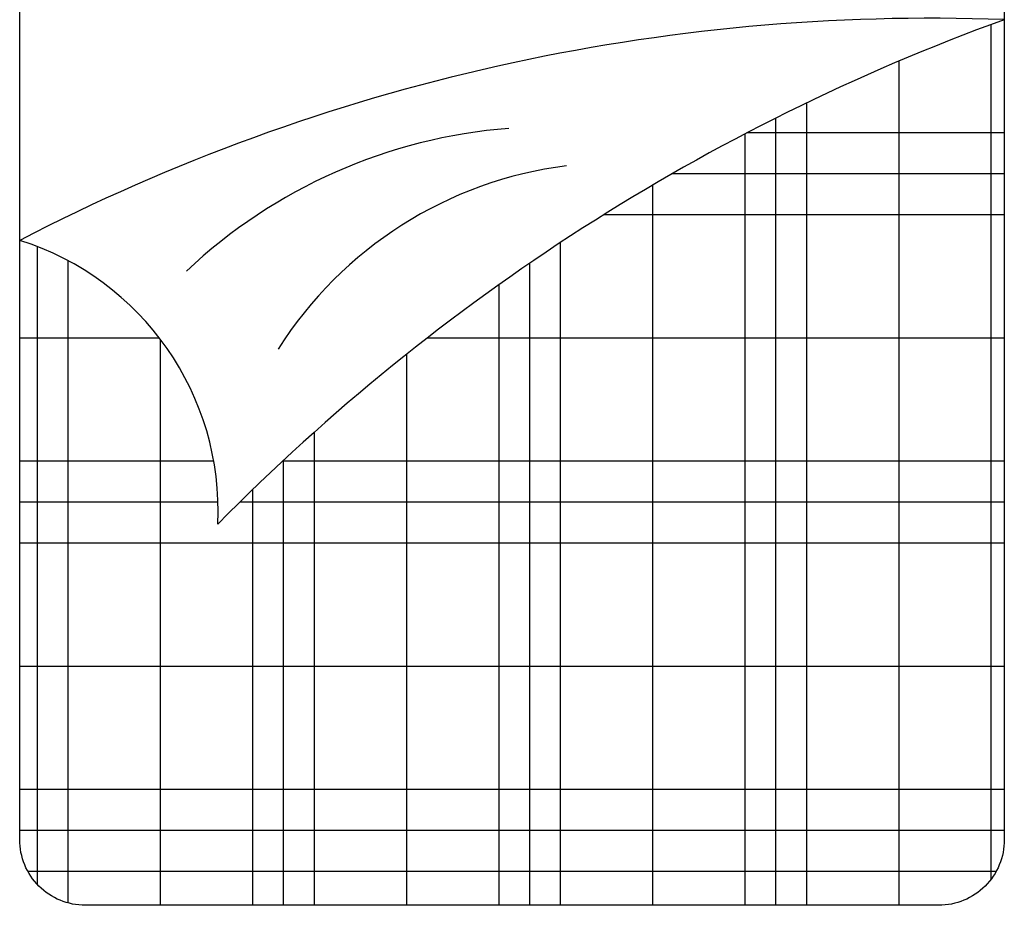
# Model space of a CAD drawing. Units: inches. Extents: x 3064 to 19385, y 846 to 15425.
# Tile 61 of 108: x 6251 to 6311, y 1911 to 1964. Entities that reach past the tile are written whole.
import ezdxf

# ---------------------------------------------------------------- set-up
doc = ezdxf.new("R2010")
doc.units = ezdxf.units.IN
doc.layers.add('A-FLOR-FIXT', color=9, linetype='Continuous', lineweight=18)
doc.layers.add('BLOCK', color=6, linetype='Continuous')

# ---------------------------------------------------------------- blocks, each defined once
blk = doc.blocks.new('*X5')
at = {"color": 0}
for p, q in [((276.598, 451.25), (280.51, 451.25)), ((275.455, 450.625), (280.51, 450.625)), ((274.411, 450), (280.51, 450)), ((265.51, 448.125), (267.634, 448.125)), ((271.723, 448.125), (280.51, 448.125)), ((265.51, 446.25), (268.465, 446.25)), ((269.519, 446.25), (280.51, 446.25)), ((265.51, 445.625), (268.531, 445.625)), ((268.866, 445.625), (280.51, 445.625)), ((265.51, 445), (280.51, 445)), ((265.51, 443.125), (280.51, 443.125)), ((265.51, 441.25), (280.51, 441.25)), ((265.51, 440.625), (280.51, 440.625)), ((265.634, 440), (280.386, 440))]:
    blk.add_line(p, q, dxfattribs=at)
blk = doc.blocks.new('*X6')
at = {"color": 0}
for p, q in [((280.312, 439.886), (280.312, 452.896)), ((278.906, 439.482), (278.906, 452.338)), ((277.5, 439.482), (277.5, 451.702)), ((277.031, 439.482), (277.031, 451.471)), ((276.562, 439.482), (276.562, 451.231)), ((275.156, 439.482), (275.156, 450.451)), ((273.75, 439.482), (273.75, 449.576)), ((265.781, 439.797), (265.781, 449.511)), ((266.25, 439.517), (266.25, 449.296)), ((273.281, 439.482), (273.281, 449.261)), ((272.812, 439.482), (272.812, 448.934)), ((267.656, 439.482), (267.656, 448.095)), ((271.406, 439.482), (271.406, 447.876)), ((270, 439.482), (270, 446.689)), ((269.531, 439.482), (269.531, 446.262)), ((269.062, 439.482), (269.062, 445.817))]:
    blk.add_line(p, q, dxfattribs=at)
blk = doc.blocks.new('A$C52E67D0D')
at = {"layer": 'BLOCK'}
blk.add_lwpolyline([(1901, 0), (601, 0, -0.414214), (501, 100), (501, 1700, -0.414214), (601, 1800), (1901, 1800, -0.414214), (2001, 1700), (2001, 100, -0.414214)], format="xyb", close=True, dxfattribs=at)
for centre, radius, start, end in [((1888.6, -1664.5), 3015.3, 87.8642, 117.4001), ((3101, -1685.8), 3227.7, 109.926, 135.3977), ((1308.8, 377.9), 807.6, 94.4436, 133.2788), ((1410.8, 520.2), 610.8, 97.2157, 147.6656), ((371.4, 600.4), 432, 357.3792, 72.5379)]:
    blk.add_arc(centre, radius, start, end, dxfattribs=at)
at = {"layer": 'BLOCK', "xscale": 100, "yscale": 100, "zscale": 100}
for name in ['*X6', '*X5']:
    blk.add_blockref(name, (-26050, -43948.2), dxfattribs=at)

msp = doc.modelspace()

# ---------------------------------------------------------------- block references
at = {"layer": 'A-FLOR-FIXT', "xscale": 0.039370099999992, "yscale": 0.039370099999992, "zscale": 0.039370099999992}
msp.add_blockref('A$C52E67D0D', (6231.741, 1911.123), dxfattribs=at)

doc.saveas('drawing.dxf')
